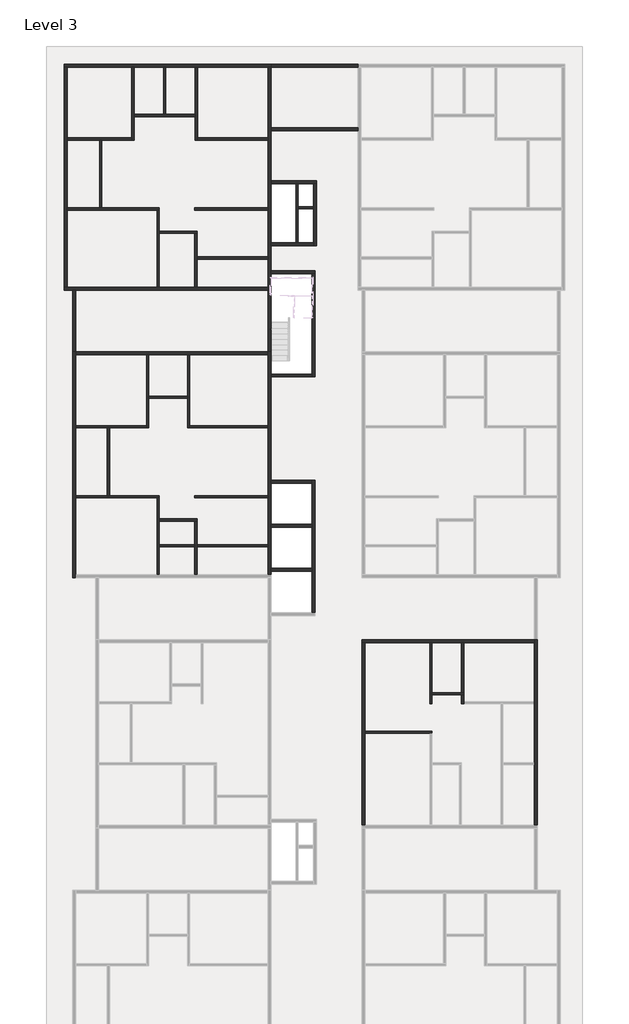
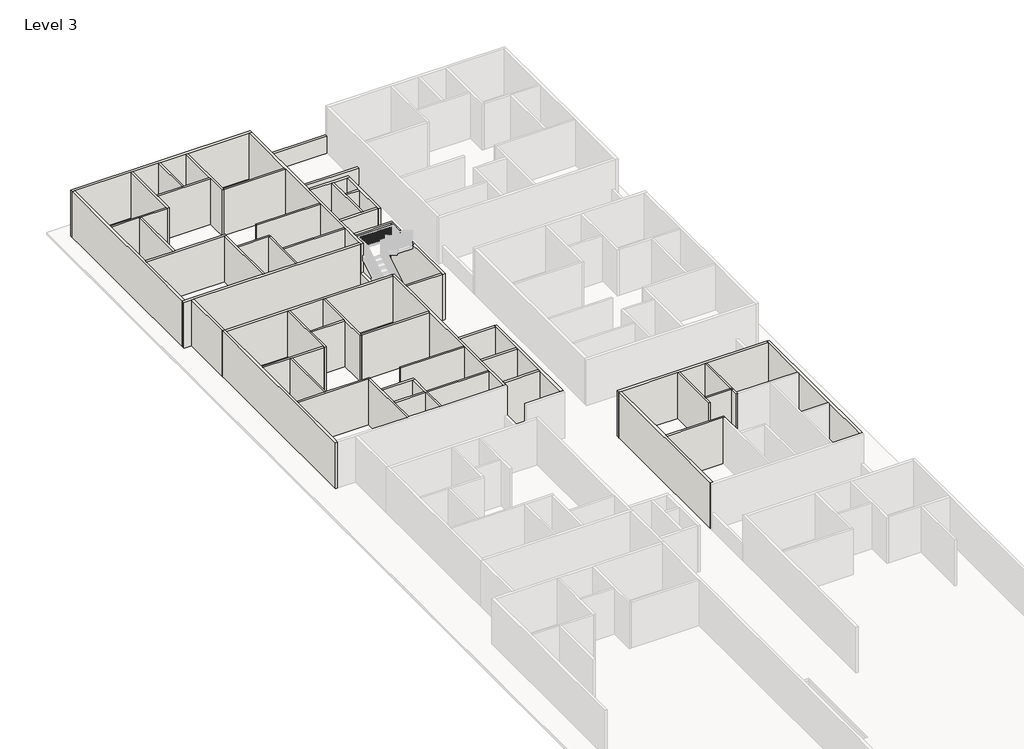
# One storey, part 3 of 8: 57 walls.
"""IFC4 building model written with IfcOpenShell, lengths in millimetres."""

from ifc_helpers import new_model, si_unit, frame, origin, place, context, project, spatial, polyline, outline, extrude, faceted_brep, element, save

model = new_model("IFC4")

# Units and contexts
model_context = context("Model", 3, world=origin())
ifc_project = project(units=[si_unit("LENGTHUNIT", "METRE", prefix="MILLI")], contexts=[model_context])

# Site, building, storey
site = spatial("IfcSite", under=ifc_project)
building = spatial("IfcBuilding", under=site)
storey = spatial("IfcBuildingStorey", under=building, Name="Level 3", Elevation=31330.6172466)

# Walls
placement = place(None, origin())
element("IfcWall", 1, ObjectType="4.5\"", at=placement, inside=storey, context=model_context, shape_type="Brep", body=[
    faceted_brep([(-10818.3415084, 35031.1216096, 31330.6172466), (-10818.3415084, 31373.5216096, 31330.6172466), (-10818.3415084, 31259.2216096, 31330.6172466), (-10818.3415084, 31259.2216096, 34378.6172466), (-10818.3415084, 31373.5216096, 34378.6172466), (-10818.3415084, 35031.1216096, 34378.6172466), (-10704.0415084, 35031.1216096, 31330.6172466), (-10704.0415084, 35031.1216096, 34378.6172466), (-10704.0415084, 32592.7216096, 34378.6172466), (-10704.0415084, 32478.4216096, 34378.6172466), (-10704.0415084, 31259.2216096, 34378.6172466), (-10704.0415084, 31259.2216096, 31330.6172466), (-10704.0415084, 32478.4216096, 31330.6172466), (-10704.0415084, 32592.7216096, 31330.6172466)], [[[0, 1, 2, 3, 4, 5]], [[6, 7, 8, 9, 10, 11, 12, 13]], [[2, 1, 0, 6, 13, 12, 11]], [[0, 5, 7, 6]], [[3, 2, 11, 10]], [[5, 4, 3, 10, 9, 8, 7]]]),
])
element("IfcWall", 2, ObjectType="4.5\"", at=placement, inside=storey, context=model_context, shape_type="Brep", body=[
    faceted_brep([(-10818.3415084, 31373.5216096, 31330.6172466), (-14171.1415084, 31373.5216096, 31330.6172466), (-14171.1415084, 31373.5216096, 34378.6172466), (-10818.3415084, 31373.5216096, 34378.6172466), (-10818.3415084, 31259.2216096, 31330.6172466), (-10818.3415084, 31259.2216096, 34378.6172466), (-12380.4415084, 31259.2216096, 34378.6172466), (-12494.7415084, 31259.2216096, 34378.6172466), (-14171.1415084, 31259.2216096, 34378.6172466), (-14171.1415084, 31259.2216096, 31330.6172466), (-12494.7415084, 31259.2216096, 31330.6172466), (-12380.4415084, 31259.2216096, 31330.6172466)], [[[0, 1, 2, 3]], [[4, 5, 6, 7, 8, 9, 10, 11]], [[1, 0, 4, 11, 10, 9]], [[0, 3, 5, 4]], [[2, 1, 9, 8]], [[3, 2, 8, 7, 6, 5]]]),
])
element("IfcWall", 3, ObjectType="4.5\"", at=placement, inside=storey, context=model_context, shape_type="SweptSolid", body=[
    extrude(outline(polyline([(-12494.7415084, 27754.0216096), (-12494.7415084, 31259.2216096), (-12380.4415084, 31259.2216096), (-12380.4415084, 27754.0216096), (-12494.7415084, 27754.0216096)])), frame((0.0, 0.0, 31330.6172466), z_axis=(0.0, 0.0, 1.0), x_axis=(1.0, 0.0, 0.0)), (0.0, 0.0, 1.0), 3048.0),
])
element("IfcWall", 4, ObjectType="4.5\"", at=placement, inside=storey, context=model_context, shape_type="Brep", body=[
    faceted_brep([(-14171.1415084, 27639.7216096, 31330.6172466), (-9510.2415084, 27639.7216096, 31330.6172466), (-9395.9415084, 27639.7216096, 31330.6172466), (-9395.9415084, 27639.7216096, 34378.6172466), (-9510.2415084, 27639.7216096, 34378.6172466), (-14171.1415084, 27639.7216096, 34378.6172466), (-14171.1415084, 27754.0216096, 31330.6172466), (-14171.1415084, 27754.0216096, 34378.6172466), (-12494.7415084, 27754.0216096, 34378.6172466), (-12380.4415084, 27754.0216096, 34378.6172466), (-9395.9415084, 27754.0216096, 34378.6172466), (-9395.9415084, 27754.0216096, 31330.6172466), (-12380.4415084, 27754.0216096, 31330.6172466), (-12494.7415084, 27754.0216096, 31330.6172466)], [[[0, 1, 2, 3, 4, 5]], [[6, 7, 8, 9, 10, 11, 12, 13]], [[2, 1, 0, 6, 13, 12, 11]], [[0, 5, 7, 6]], [[3, 2, 11, 10]], [[5, 4, 3, 10, 9, 8, 7]]]),
])
element("IfcWall", 5, ObjectType="4.5\"", at=placement, inside=storey, context=model_context, shape_type="Brep", body=[
    faceted_brep([(-9510.2415084, 27639.7216096, 31330.6172466), (-9510.2415084, 23651.9216096, 31330.6172466), (-9510.2415084, 23651.9216096, 34378.6172466), (-9510.2415084, 27639.7216096, 34378.6172466), (-9395.9415084, 27639.7216096, 31330.6172466), (-9395.9415084, 27639.7216096, 34378.6172466), (-9395.9415084, 26547.5216096, 34378.6172466), (-9395.9415084, 26433.2216096, 34378.6172466), (-9395.9415084, 23651.9216096, 34378.6172466), (-9395.9415084, 23651.9216096, 31330.6172466), (-9395.9415084, 26433.2216096, 31330.6172466), (-9395.9415084, 26547.5216096, 31330.6172466)], [[[0, 1, 2, 3]], [[4, 5, 6, 7, 8, 9, 10, 11]], [[1, 0, 4, 11, 10, 9]], [[0, 3, 5, 4]], [[2, 1, 9, 8]], [[3, 2, 8, 7, 6, 5]]]),
])
element("IfcWall", 6, ObjectType="4.5\"", at=placement, inside=storey, context=model_context, shape_type="Brep", body=[
    faceted_brep([(-9395.9415084, 26433.2216096, 31330.6172466), (-7567.1415084, 26433.2216096, 31330.6172466), (-7452.8415084, 26433.2216096, 31330.6172466), (-7452.8415084, 26433.2216096, 34378.6172466), (-7567.1415084, 26433.2216096, 34378.6172466), (-9395.9415084, 26433.2216096, 34378.6172466), (-9395.9415084, 26547.5216096, 31330.6172466), (-9395.9415084, 26547.5216096, 34378.6172466), (-7452.8415084, 26547.5216096, 34378.6172466), (-7452.8415084, 26547.5216096, 31330.6172466)], [[[0, 1, 2, 3, 4, 5]], [[6, 7, 8, 9]], [[2, 1, 0, 6, 9]], [[0, 5, 7, 6]], [[3, 2, 9, 8]], [[5, 4, 3, 8, 7]]]),
])
element("IfcWall", 7, ObjectType="4.5\"", at=placement, inside=storey, context=model_context, shape_type="Brep", body=[
    faceted_brep([(-7567.1415084, 26433.2216096, 31330.6172466), (-7567.1415084, 23651.9216096, 31330.6172466), (-7567.1415084, 23651.9216096, 34378.6172466), (-7567.1415084, 26433.2216096, 34378.6172466), (-7452.8415084, 26433.2216096, 31330.6172466), (-7452.8415084, 26433.2216096, 34378.6172466), (-7452.8415084, 25214.0216096, 34378.6172466), (-7452.8415084, 25099.7216096, 34378.6172466), (-7452.8415084, 23651.9216096, 34378.6172466), (-7452.8415084, 23651.9216096, 31330.6172466), (-7452.8415084, 25099.7216096, 31330.6172466), (-7452.8415084, 25214.0216096, 31330.6172466)], [[[0, 1, 2, 3]], [[4, 5, 6, 7, 8, 9, 10, 11]], [[1, 0, 4, 11, 10, 9]], [[0, 3, 5, 4]], [[2, 1, 9, 8]], [[3, 2, 8, 7, 6, 5]]]),
])
element("IfcWall", 8, ObjectType="4.5\"", at=placement, inside=storey, context=model_context, shape_type="SweptSolid", body=[
    extrude(outline(polyline([(-7452.8415084, 25214.0216096), (-3769.8415084, 25214.0216096), (-3769.8415084, 25099.7216096), (-7452.8415084, 25099.7216096), (-7452.8415084, 25214.0216096)])), frame((0.0, 0.0, 31330.6172466), z_axis=(0.0, 0.0, 1.0), x_axis=(1.0, 0.0, 0.0)), (0.0, 0.0, 1.0), 3048.0),
])
element("IfcWall", 9, ObjectType="4.5\"", at=placement, inside=storey, context=model_context, shape_type="SweptSolid", body=[
    extrude(outline(polyline([(-3769.8415084, 27639.7216096), (-7567.1415084, 27639.7216096), (-7567.1415084, 27754.0216096), (-3769.8415084, 27754.0216096), (-3769.8415084, 27639.7216096)])), frame((0.0, 0.0, 31330.6172466), z_axis=(0.0, 0.0, 1.0), x_axis=(1.0, 0.0, 0.0)), (0.0, 0.0, 1.0), 3048.0),
])
element("IfcWall", 10, ObjectType="4.5\"", at=placement, inside=storey, context=model_context, shape_type="Brep", body=[
    faceted_brep([(-10704.0415084, 32478.4216096, 31330.6172466), (-7541.7415084, 32478.4216096, 31330.6172466), (-7541.7415084, 32478.4216096, 34378.6172466), (-10704.0415084, 32478.4216096, 34378.6172466), (-10704.0415084, 32592.7216096, 31330.6172466), (-10704.0415084, 32592.7216096, 34378.6172466), (-9180.0415084, 32592.7216096, 34378.6172466), (-9065.7415084, 32592.7216096, 34378.6172466), (-7541.7415084, 32592.7216096, 34378.6172466), (-7541.7415084, 32592.7216096, 31330.6172466), (-9065.7415084, 32592.7216096, 31330.6172466), (-9180.0415084, 32592.7216096, 31330.6172466)], [[[0, 1, 2, 3]], [[4, 5, 6, 7, 8, 9, 10, 11]], [[1, 0, 4, 11, 10, 9]], [[0, 3, 5, 4]], [[2, 1, 9, 8]], [[3, 2, 8, 7, 6, 5]]]),
])
element("IfcWall", 11, ObjectType="4.5\"", at=placement, inside=storey, context=model_context, shape_type="SweptSolid", body=[
    extrude(outline(polyline([(-9180.0415084, 32592.7216096), (-9180.0415084, 35031.1216096), (-9065.7415084, 35031.1216096), (-9065.7415084, 32592.7216096), (-9180.0415084, 32592.7216096)])), frame((0.0, 0.0, 31330.6172466), z_axis=(0.0, 0.0, 1.0), x_axis=(1.0, 0.0, 0.0)), (0.0, 0.0, 1.0), 3048.0),
])
element("IfcWall", 12, ObjectType="4.5\"", at=placement, inside=storey, context=model_context, shape_type="Brep", body=[
    faceted_brep([(-7541.7415084, 35031.1216096, 31330.6172466), (-7541.7415084, 32592.7216096, 31330.6172466), (-7541.7415084, 32478.4216096, 31330.6172466), (-7541.7415084, 31259.2216096, 31330.6172466), (-7541.7415084, 31259.2216096, 34378.6172466), (-7541.7415084, 32478.4216096, 34378.6172466), (-7541.7415084, 32592.7216096, 34378.6172466), (-7541.7415084, 35031.1216096, 34378.6172466), (-7427.4415084, 35031.1216096, 31330.6172466), (-7427.4415084, 35031.1216096, 34378.6172466), (-7427.4415084, 31373.5216096, 34378.6172466), (-7427.4415084, 31259.2216096, 34378.6172466), (-7427.4415084, 31259.2216096, 31330.6172466), (-7427.4415084, 31373.5216096, 31330.6172466)], [[[0, 1, 2, 3, 4, 5, 6, 7]], [[8, 9, 10, 11, 12, 13]], [[3, 2, 1, 0, 8, 13, 12]], [[0, 7, 9, 8]], [[4, 3, 12, 11]], [[7, 6, 5, 4, 11, 10, 9]]]),
])
element("IfcWall", 13, ObjectType="4.5\"", at=placement, inside=storey, context=model_context, shape_type="SweptSolid", body=[
    extrude(outline(polyline([(-3769.8415084, 31259.2216096), (-7427.4415084, 31259.2216096), (-7427.4415084, 31373.5216096), (-3769.8415084, 31373.5216096), (-3769.8415084, 31259.2216096)])), frame((0.0, 0.0, 31330.6172466), z_axis=(0.0, 0.0, 1.0), x_axis=(1.0, 0.0, 0.0)), (0.0, 0.0, 1.0), 3048.0),
])
element("IfcWall", 14, ObjectType="4.5\"", at=placement, inside=storey, context=model_context, shape_type="Brep", body=[
    faceted_brep([(-10061.4044854, 20146.7216096, 31330.6172466), (-10061.4044854, 16489.1216096, 31330.6172466), (-10061.4044854, 16374.8216096, 31330.6172466), (-10061.4044854, 16374.8216096, 34378.6172466), (-10061.4044854, 16489.1216096, 34378.6172466), (-10061.4044854, 20146.7216096, 34378.6172466), (-9947.1044854, 20146.7216096, 31330.6172466), (-9947.1044854, 20146.7216096, 34378.6172466), (-9947.1044854, 18013.1216096, 34378.6172466), (-9947.1044854, 17898.8216096, 34378.6172466), (-9947.1044854, 16374.8216096, 34378.6172466), (-9947.1044854, 16374.8216096, 31330.6172466), (-9947.1044854, 17898.8216096, 31330.6172466), (-9947.1044854, 18013.1216096, 31330.6172466)], [[[0, 1, 2, 3, 4, 5]], [[6, 7, 8, 9, 10, 11, 12, 13]], [[2, 1, 0, 6, 13, 12, 11]], [[0, 5, 7, 6]], [[3, 2, 11, 10]], [[5, 4, 3, 10, 9, 8, 7]]]),
])
element("IfcWall", 15, ObjectType="4.5\"", at=placement, inside=storey, context=model_context, shape_type="Brep", body=[
    faceted_brep([(-10061.4044854, 16489.1216096, 31330.6172466), (-13719.0044854, 16489.1216096, 31330.6172466), (-13719.0044854, 16489.1216096, 34378.6172466), (-10061.4044854, 16489.1216096, 34378.6172466), (-10061.4044854, 16374.8216096, 31330.6172466), (-10061.4044854, 16374.8216096, 34378.6172466), (-11980.3915084, 16374.8216096, 34378.6172466), (-12094.6915084, 16374.8216096, 34378.6172466), (-13719.0044854, 16374.8216096, 34378.6172466), (-13719.0044854, 16374.8216096, 31330.6172466), (-12094.6915084, 16374.8216096, 31330.6172466), (-11980.3915084, 16374.8216096, 31330.6172466)], [[[0, 1, 2, 3]], [[4, 5, 6, 7, 8, 9, 10, 11]], [[1, 0, 4, 11, 10, 9]], [[0, 3, 5, 4]], [[2, 1, 9, 8]], [[3, 2, 8, 7, 6, 5]]]),
])
element("IfcWall", 16, ObjectType="4.5\"", at=placement, inside=storey, context=model_context, shape_type="SweptSolid", body=[
    extrude(outline(polyline([(-7940.5044854, 17898.8216096), (-9947.1044854, 17898.8216096), (-9947.1044854, 18013.1216096), (-7940.5044854, 18013.1216096), (-7940.5044854, 17898.8216096)])), frame((0.0, 0.0, 31330.6172466), z_axis=(0.0, 0.0, 1.0), x_axis=(1.0, 0.0, 0.0)), (0.0, 0.0, 1.0), 3048.0),
])
element("IfcWall", 17, ObjectType="4.5\"", at=placement, inside=storey, context=model_context, shape_type="Brep", body=[
    faceted_brep([(-7940.5044854, 20146.7216096, 31330.6172466), (-7940.5044854, 18013.1216096, 31330.6172466), (-7940.5044854, 17898.8216096, 31330.6172466), (-7940.5044854, 16374.8216096, 31330.6172466), (-7940.5044854, 16374.8216096, 34378.6172466), (-7940.5044854, 17898.8216096, 34378.6172466), (-7940.5044854, 18013.1216096, 34378.6172466), (-7940.5044854, 20146.7216096, 34378.6172466), (-7826.2044854, 20146.7216096, 31330.6172466), (-7826.2044854, 20146.7216096, 34378.6172466), (-7826.2044854, 16489.1216096, 34378.6172466), (-7826.2044854, 16374.8216096, 34378.6172466), (-7826.2044854, 16374.8216096, 31330.6172466), (-7826.2044854, 16489.1216096, 31330.6172466)], [[[0, 1, 2, 3, 4, 5, 6, 7]], [[8, 9, 10, 11, 12, 13]], [[3, 2, 1, 0, 8, 13, 12]], [[0, 7, 9, 8]], [[4, 3, 12, 11]], [[7, 6, 5, 4, 11, 10, 9]]]),
])
element("IfcWall", 18, ObjectType="4.5\"", at=placement, inside=storey, context=model_context, shape_type="SweptSolid", body=[
    extrude(outline(polyline([(-3769.8415084, 16374.8216096), (-7826.2044854, 16374.8216096), (-7826.2044854, 16489.1216096), (-3769.8415084, 16489.1216096), (-3769.8415084, 16374.8216096)])), frame((0.0, 0.0, 31330.6172466), z_axis=(0.0, 0.0, 1.0), x_axis=(1.0, 0.0, 0.0)), (0.0, 0.0, 1.0), 3048.0),
])
element("IfcWall", 19, ObjectType="4.5\"", at=placement, inside=storey, context=model_context, shape_type="SweptSolid", body=[
    extrude(outline(polyline([(-12094.6915084, 12869.6216096), (-12094.6915084, 16374.8216096), (-11980.3915084, 16374.8216096), (-11980.3915084, 12869.6216096), (-12094.6915084, 12869.6216096)])), frame((0.0, 0.0, 31330.6172466), z_axis=(0.0, 0.0, 1.0), x_axis=(1.0, 0.0, 0.0)), (0.0, 0.0, 1.0), 3048.0),
])
element("IfcWall", 20, ObjectType="4.5\"", at=placement, inside=storey, context=model_context, shape_type="Brep", body=[
    faceted_brep([(-13719.0044854, 12755.3216096, 31330.6172466), (-9510.2415084, 12755.3216096, 31330.6172466), (-9395.9415084, 12755.3216096, 31330.6172466), (-9395.9415084, 12755.3216096, 34378.6172466), (-9510.2415084, 12755.3216096, 34378.6172466), (-13719.0044854, 12755.3216096, 34378.6172466), (-13719.0044854, 12869.6216096, 31330.6172466), (-13719.0044854, 12869.6216096, 34378.6172466), (-12094.6915084, 12869.6216096, 34378.6172466), (-11980.3915084, 12869.6216096, 34378.6172466), (-9395.9415084, 12869.6216096, 34378.6172466), (-9395.9415084, 12869.6216096, 31330.6172466), (-11980.3915084, 12869.6216096, 31330.6172466), (-12094.6915084, 12869.6216096, 31330.6172466)], [[[0, 1, 2, 3, 4, 5]], [[6, 7, 8, 9, 10, 11, 12, 13]], [[2, 1, 0, 6, 13, 12, 11]], [[0, 5, 7, 6]], [[3, 2, 11, 10]], [[5, 4, 3, 10, 9, 8, 7]]]),
])
element("IfcWall", 21, ObjectType="4.5\"", at=placement, inside=storey, context=model_context, shape_type="Brep", body=[
    faceted_brep([(-9510.2415084, 12755.3216096, 31330.6172466), (-9510.2415084, 8767.5216096, 31330.6172466), (-9510.2415084, 8767.5216096, 34378.6172466), (-9510.2415084, 12755.3216096, 34378.6172466), (-9395.9415084, 12755.3216096, 31330.6172466), (-9395.9415084, 12755.3216096, 34378.6172466), (-9395.9415084, 11663.1216096, 34378.6172466), (-9395.9415084, 11548.8216096, 34378.6172466), (-9395.9415084, 10329.6216096, 34378.6172466), (-9395.9415084, 10215.3216096, 34378.6172466), (-9395.9415084, 8767.5216096, 34378.6172466), (-9395.9415084, 8767.5216096, 31330.6172466), (-9395.9415084, 10215.3216096, 31330.6172466), (-9395.9415084, 10329.6216096, 31330.6172466), (-9395.9415084, 11548.8216096, 31330.6172466), (-9395.9415084, 11663.1216096, 31330.6172466)], [[[0, 1, 2, 3]], [[4, 5, 6, 7, 8, 9, 10, 11, 12, 13, 14, 15]], [[1, 0, 4, 15, 14, 13, 12, 11]], [[0, 3, 5, 4]], [[2, 1, 11, 10]], [[3, 2, 10, 9, 8, 7, 6, 5]]]),
])
element("IfcWall", 22, ObjectType="4.5\"", at=placement, inside=storey, context=model_context, shape_type="SweptSolid", body=[
    extrude(outline(polyline([(-7567.1415084, 10215.3216096), (-9395.9415084, 10215.3216096), (-9395.9415084, 10329.6216096), (-7567.1415084, 10329.6216096), (-7567.1415084, 10215.3216096)])), frame((0.0, 0.0, 31330.6172466), z_axis=(0.0, 0.0, 1.0), x_axis=(1.0, 0.0, 0.0)), (0.0, 0.0, 1.0), 3048.0),
])
element("IfcWall", 23, ObjectType="4.5\"", at=placement, inside=storey, context=model_context, shape_type="Brep", body=[
    faceted_brep([(-9395.9415084, 11548.8216096, 31330.6172466), (-7567.1415084, 11548.8216096, 31330.6172466), (-7452.8415084, 11548.8216096, 31330.6172466), (-7452.8415084, 11548.8216096, 34378.6172466), (-7567.1415084, 11548.8216096, 34378.6172466), (-9395.9415084, 11548.8216096, 34378.6172466), (-9395.9415084, 11663.1216096, 31330.6172466), (-9395.9415084, 11663.1216096, 34378.6172466), (-7452.8415084, 11663.1216096, 34378.6172466), (-7452.8415084, 11663.1216096, 31330.6172466)], [[[0, 1, 2, 3, 4, 5]], [[6, 7, 8, 9]], [[2, 1, 0, 6, 9]], [[0, 5, 7, 6]], [[3, 2, 9, 8]], [[5, 4, 3, 8, 7]]]),
])
element("IfcWall", 24, ObjectType="4.5\"", at=placement, inside=storey, context=model_context, shape_type="Brep", body=[
    faceted_brep([(-7567.1415084, 11548.8216096, 31330.6172466), (-7567.1415084, 10329.6216096, 31330.6172466), (-7567.1415084, 10215.3216096, 31330.6172466), (-7567.1415084, 8767.5216096, 31330.6172466), (-7567.1415084, 8767.5216096, 34378.6172466), (-7567.1415084, 10215.3216096, 34378.6172466), (-7567.1415084, 10329.6216096, 34378.6172466), (-7567.1415084, 11548.8216096, 34378.6172466), (-7452.8415084, 11548.8216096, 31330.6172466), (-7452.8415084, 11548.8216096, 34378.6172466), (-7452.8415084, 10329.6216096, 34378.6172466), (-7452.8415084, 10215.3216096, 34378.6172466), (-7452.8415084, 8767.5216096, 34378.6172466), (-7452.8415084, 8767.5216096, 31330.6172466), (-7452.8415084, 10215.3216096, 31330.6172466), (-7452.8415084, 10329.6216096, 31330.6172466)], [[[0, 1, 2, 3, 4, 5, 6, 7]], [[8, 9, 10, 11, 12, 13, 14, 15]], [[3, 2, 1, 0, 8, 15, 14, 13]], [[0, 7, 9, 8]], [[4, 3, 13, 12]], [[7, 6, 5, 4, 12, 11, 10, 9]]]),
])
element("IfcWall", 25, ObjectType="4.5\"", at=placement, inside=storey, context=model_context, shape_type="SweptSolid", body=[
    extrude(outline(polyline([(-3769.8415084, 10215.3216096), (-7452.8415084, 10215.3216096), (-7452.8415084, 10329.6216096), (-3769.8415084, 10329.6216096), (-3769.8415084, 10215.3216096)])), frame((0.0, 0.0, 31330.6172466), z_axis=(0.0, 0.0, 1.0), x_axis=(1.0, 0.0, 0.0)), (0.0, 0.0, 1.0), 3048.0),
])
element("IfcWall", 26, ObjectType="4.5\"", at=placement, inside=storey, context=model_context, shape_type="SweptSolid", body=[
    extrude(outline(polyline([(-3769.8415084, 12755.3216096), (-7567.1415084, 12755.3216096), (-7567.1415084, 12869.6216096), (-3769.8415084, 12869.6216096), (-3769.8415084, 12755.3216096)])), frame((0.0, 0.0, 31330.6172466), z_axis=(0.0, 0.0, 1.0), x_axis=(1.0, 0.0, 0.0)), (0.0, 0.0, 1.0), 3048.0),
])
element("IfcWall", 27, ObjectType="4.5\"", at=placement, inside=storey, context=model_context, shape_type="Brep", body=[
    faceted_brep([(1259.3584916, 572.7745083, 31330.6172466), (4610.8714687, 572.7745083, 31330.6172466), (4725.1714687, 572.7745083, 31330.6172466), (4725.1714687, 572.7745083, 34378.6172466), (4610.8714687, 572.7745083, 34378.6172466), (1259.3584916, 572.7745083, 34378.6172466), (1259.3584916, 687.0745083, 31330.6172466), (1259.3584916, 687.0745083, 34378.6172466), (4725.1714687, 687.0745083, 34378.6172466), (4725.1714687, 687.0745083, 31330.6172466)], [[[0, 1, 2, 3, 4, 5]], [[6, 7, 8, 9]], [[2, 1, 0, 6, 9]], [[0, 5, 7, 6]], [[3, 2, 9, 8]], [[5, 4, 3, 8, 7]]]),
])
element("IfcWall", 28, ObjectType="4.5\"", at=placement, inside=storey, context=model_context, shape_type="Brep", body=[
    faceted_brep([(4610.8714687, 5262.3216096, 31330.6172466), (4610.8714687, 2100.0216096, 31330.6172466), (4610.8714687, 2100.0216096, 34378.6172466), (4610.8714687, 5262.3216096, 34378.6172466), (4725.1714687, 5262.3216096, 31330.6172466), (4725.1714687, 5262.3216096, 34378.6172466), (4725.1714687, 2671.5216096, 34378.6172466), (4725.1714687, 2557.2216096, 34378.6172466), (4725.1714687, 2100.0216096, 34378.6172466), (4725.1714687, 2100.0216096, 31330.6172466), (4725.1714687, 2557.2216096, 31330.6172466), (4725.1714687, 2671.5216096, 31330.6172466)], [[[0, 1, 2, 3]], [[4, 5, 6, 7, 8, 9, 10, 11]], [[1, 0, 4, 11, 10, 9]], [[2, 1, 9, 8]], [[0, 3, 5, 4]], [[3, 2, 8, 7, 6, 5]]]),
])
element("IfcWall", 29, ObjectType="4.5\"", at=placement, inside=storey, context=model_context, shape_type="Brep", body=[
    faceted_brep([(4725.1714687, 2557.2216096, 31330.6172466), (6249.1714687, 2557.2216096, 31330.6172466), (6363.4714687, 2557.2216096, 31330.6172466), (6363.4714687, 2557.2216096, 34378.6172466), (6249.1714687, 2557.2216096, 34378.6172466), (4725.1714687, 2557.2216096, 34378.6172466), (4725.1714687, 2671.5216096, 31330.6172466), (4725.1714687, 2671.5216096, 34378.6172466), (6249.1714687, 2671.5216096, 34378.6172466), (6363.4714687, 2671.5216096, 34378.6172466), (6363.4714687, 2671.5216096, 31330.6172466), (6249.1714687, 2671.5216096, 31330.6172466)], [[[0, 1, 2, 3, 4, 5]], [[6, 7, 8, 9, 10, 11]], [[2, 1, 0, 6, 11, 10]], [[0, 5, 7, 6]], [[3, 2, 10, 9]], [[5, 4, 3, 9, 8, 7]]]),
])
element("IfcWall", 30, ObjectType="4.5\"", at=placement, inside=storey, context=model_context, shape_type="SweptSolid", body=[
    extrude(outline(polyline([(6363.4714687, 5262.3216096), (6363.4714687, 2671.5216096), (6249.1714687, 2671.5216096), (6249.1714687, 5262.3216096), (6363.4714687, 5262.3216096)])), frame((0.0, 0.0, 31330.6172466), z_axis=(0.0, 0.0, 1.0), x_axis=(1.0, 0.0, 0.0)), (0.0, 0.0, 1.0), 3048.0),
])
element("IfcWall", 31, ObjectType="4.5\"", at=placement, inside=storey, context=model_context, shape_type="Brep", body=[
    faceted_brep([(6249.1714687, 2557.2216096, 31330.6172466), (6249.1714687, 2100.0216096, 31330.6172466), (6249.1714687, 2100.0216096, 34378.6172466), (6249.1714687, 2557.2216096, 34378.6172466), (6363.4714687, 2557.2216096, 31330.6172466), (6363.4714687, 2557.2216096, 34378.6172466), (6363.4714687, 2214.3216096, 34378.6172466), (6363.4714687, 2100.0216096, 34378.6172466), (6363.4714687, 2100.0216096, 31330.6172466), (6363.4714687, 2214.3216096, 31330.6172466)], [[[0, 1, 2, 3]], [[4, 5, 6, 7, 8, 9]], [[1, 0, 4, 9, 8]], [[0, 3, 5, 4]], [[2, 1, 8, 7]], [[3, 2, 7, 6, 5]]]),
])
element("IfcWall", 32, ObjectType="4.5\"", at=placement, inside=storey, context=model_context, shape_type="Brep", body=[
    faceted_brep([(-2321.9738684, 29000.0900967, 31330.6172466), (-2321.9738684, 25952.0900967, 31330.6172466), (-2321.9738684, 25952.0900967, 34378.6172466), (-2321.9738684, 29000.0900967, 34378.6172466), (-2207.6738684, 29000.0900967, 31330.6172466), (-2207.6738684, 29000.0900967, 34378.6172466), (-2207.6738684, 27820.8172885, 34378.6172466), (-2207.6738684, 27706.5172885, 34378.6172466), (-2207.6738684, 25952.0900967, 34378.6172466), (-2207.6738684, 25952.0900967, 31330.6172466), (-2207.6738684, 27706.5172885, 31330.6172466), (-2207.6738684, 27820.8172885, 31330.6172466)], [[[0, 1, 2, 3]], [[4, 5, 6, 7, 8, 9, 10, 11]], [[1, 0, 4, 11, 10, 9]], [[3, 2, 8, 7, 6, 5]], [[0, 3, 5, 4]], [[2, 1, 9, 8]]]),
])
element("IfcWall", 33, ObjectType="4.5\"", at=placement, inside=storey, context=model_context, shape_type="SweptSolid", body=[
    extrude(outline(polyline([(-2207.6738684, 27820.8172885), (-1407.6415084, 27820.8172885), (-1407.6415084, 27706.5172885), (-2207.6738684, 27706.5172885), (-2207.6738684, 27820.8172885)])), frame((0.0, 0.0, 31330.6172466), z_axis=(0.0, 0.0, 1.0), x_axis=(1.0, 0.0, 0.0)), (0.0, 0.0, 1.0), 3048.0),
])
element("IfcWall", 34, ObjectType="6\"", at=placement, inside=storey, context=model_context, shape_type="Brep", body=[
    faceted_brep([(-14323.5415084, 35031.1216096, 31330.6172466), (-14171.1415084, 35031.1216096, 31330.6172466), (-10818.3415084, 35031.1216096, 31330.6172466), (-10704.0415084, 35031.1216096, 31330.6172466), (-9180.0415084, 35031.1216096, 31330.6172466), (-9065.7415084, 35031.1216096, 31330.6172466), (-7541.7415084, 35031.1216096, 31330.6172466), (-7427.4415084, 35031.1216096, 31330.6172466), (-3769.8415084, 35031.1216096, 31330.6172466), (-3617.4415084, 35031.1216096, 31330.6172466), (-3617.4415084, 35031.1216096, 34378.6172466), (-3769.8415084, 35031.1216096, 34378.6172466), (-7427.4415084, 35031.1216096, 34378.6172466), (-7541.7415084, 35031.1216096, 34378.6172466), (-9065.7415084, 35031.1216096, 34378.6172466), (-9180.0415084, 35031.1216096, 34378.6172466), (-10704.0415084, 35031.1216096, 34378.6172466), (-10818.3415084, 35031.1216096, 34378.6172466), (-14171.1415084, 35031.1216096, 34378.6172466), (-14323.5415084, 35031.1216096, 34378.6172466), (-14323.5415084, 35183.5216096, 31330.6172466), (-14323.5415084, 35183.5216096, 34378.6172466), (-3617.4415084, 35183.5216096, 34378.6172466), (-3617.4415084, 35183.5216096, 31330.6172466)], [[[0, 1, 2, 3, 4, 5, 6, 7, 8, 9, 10, 11, 12, 13, 14, 15, 16, 17, 18, 19]], [[20, 21, 22, 23]], [[9, 8, 7, 6, 5, 4, 3, 2, 1, 0, 20, 23]], [[0, 19, 21, 20]], [[9, 23, 22, 10]], [[19, 18, 17, 16, 15, 14, 13, 12, 11, 10, 22, 21]]]),
])
element("IfcWall", 35, ObjectType="6\"", at=placement, inside=storey, context=model_context, shape_type="Brep", body=[
    faceted_brep([(-3769.8415084, 35031.1216096, 34378.6172466), (-3769.8415084, 35031.1216096, 31330.6172466), (-3769.8415084, 31373.5216096, 31330.6172466), (-3769.8415084, 31259.2216096, 31330.6172466), (-3769.8415084, 27754.0216096, 31330.6172466), (-3769.8415084, 27639.7216096, 31330.6172466), (-3769.8415084, 25214.0216096, 31330.6172466), (-3769.8415084, 25099.7216096, 31330.6172466), (-3769.8415084, 23651.9216096, 31330.6172466), (-3769.8415084, 23499.5216096, 31330.6172466), (-3769.8415084, 23499.5216096, 34378.6172466), (-3769.8415084, 23651.9216096, 34378.6172466), (-3769.8415084, 25099.7216096, 34378.6172466), (-3769.8415084, 25214.0216096, 34378.6172466), (-3769.8415084, 27639.7216096, 34378.6172466), (-3769.8415084, 27754.0216096, 34378.6172466), (-3769.8415084, 31259.2216096, 34378.6172466), (-3769.8415084, 31373.5216096, 34378.6172466), (-3617.4415084, 35031.1216096, 31330.6172466), (-3617.4415084, 35031.1216096, 34378.6172466), (-3617.4415084, 29152.4900967, 34378.6172466), (-3617.4415084, 29000.0900967, 34378.6172466), (-3617.4415084, 25952.0900967, 34378.6172466), (-3617.4415084, 25799.6900967, 34378.6172466), (-3617.4415084, 24490.1216096, 34378.6172466), (-3617.4415084, 24337.7216096, 34378.6172466), (-3617.4415084, 23499.5216096, 34378.6172466), (-3617.4415084, 23499.5216096, 31330.6172466), (-3617.4415084, 24337.7216096, 31330.6172466), (-3617.4415084, 24490.1216096, 31330.6172466), (-3617.4415084, 25799.6900967, 31330.6172466), (-3617.4415084, 25952.0900967, 31330.6172466), (-3617.4415084, 29000.0900967, 31330.6172466), (-3617.4415084, 29152.4900967, 31330.6172466), (-3617.4415084, 31744.9197155, 31330.6172466), (-3617.4415084, 31897.3197155, 31330.6172466)], [[[0, 1, 2, 3, 4, 5, 6, 7, 8, 9, 10, 11, 12, 13, 14, 15, 16, 17]], [[18, 19, 20, 21, 22, 23, 24, 25, 26, 27, 28, 29, 30, 31, 32, 33, 34, 35]], [[9, 8, 7, 6, 5, 4, 3, 2, 1, 18, 35, 34, 33, 32, 31, 30, 29, 28, 27]], [[0, 19, 18, 1]], [[9, 27, 26, 10]], [[0, 17, 16, 15, 14, 13, 12, 11, 10, 26, 25, 24, 23, 22, 21, 20, 19]]]),
])
element("IfcWall", 36, ObjectType="6\"", at=placement, inside=storey, context=model_context, shape_type="Brep", body=[
    faceted_brep([(-3769.8415084, 23651.9216096, 34378.6172466), (-3769.8415084, 23651.9216096, 31330.6172466), (-7452.8415084, 23651.9216096, 31330.6172466), (-7567.1415084, 23651.9216096, 31330.6172466), (-9395.9415084, 23651.9216096, 31330.6172466), (-9510.2415084, 23651.9216096, 31330.6172466), (-14171.1415084, 23651.9216096, 31330.6172466), (-14323.5415084, 23651.9216096, 31330.6172466), (-14323.5415084, 23651.9216096, 34378.6172466), (-14171.1415084, 23651.9216096, 34378.6172466), (-9510.2415084, 23651.9216096, 34378.6172466), (-9395.9415084, 23651.9216096, 34378.6172466), (-7567.1415084, 23651.9216096, 34378.6172466), (-7452.8415084, 23651.9216096, 34378.6172466), (-3769.8415084, 23499.5216096, 31330.6172466), (-3769.8415084, 23499.5216096, 34378.6172466), (-13719.0044854, 23499.5216096, 34378.6172466), (-13871.4044854, 23499.5216096, 34378.6172466), (-14323.5415084, 23499.5216096, 34378.6172466), (-14323.5415084, 23499.5216096, 31330.6172466), (-13871.4044854, 23499.5216096, 31330.6172466), (-13719.0044854, 23499.5216096, 31330.6172466)], [[[0, 1, 2, 3, 4, 5, 6, 7, 8, 9, 10, 11, 12, 13]], [[14, 15, 16, 17, 18, 19, 20, 21]], [[7, 6, 5, 4, 3, 2, 1, 14, 21, 20, 19]], [[8, 7, 19, 18]], [[0, 15, 14, 1]], [[0, 13, 12, 11, 10, 9, 8, 18, 17, 16, 15]]]),
])
element("IfcWall", 37, ObjectType="6\"", at=placement, inside=storey, context=model_context, shape_type="Brep", body=[
    faceted_brep([(-14171.1415084, 23651.9216096, 31330.6172466), (-14171.1415084, 27639.7216096, 31330.6172466), (-14171.1415084, 27754.0216096, 31330.6172466), (-14171.1415084, 31259.2216096, 31330.6172466), (-14171.1415084, 31373.5216096, 31330.6172466), (-14171.1415084, 35031.1216096, 31330.6172466), (-14171.1415084, 35031.1216096, 34378.6172466), (-14171.1415084, 31373.5216096, 34378.6172466), (-14171.1415084, 31259.2216096, 34378.6172466), (-14171.1415084, 27754.0216096, 34378.6172466), (-14171.1415084, 27639.7216096, 34378.6172466), (-14171.1415084, 23651.9216096, 34378.6172466), (-14323.5415084, 23651.9216096, 31330.6172466), (-14323.5415084, 23651.9216096, 34378.6172466), (-14323.5415084, 35031.1216096, 34378.6172466), (-14323.5415084, 35031.1216096, 31330.6172466)], [[[0, 1, 2, 3, 4, 5, 6, 7, 8, 9, 10, 11]], [[12, 13, 14, 15]], [[5, 4, 3, 2, 1, 0, 12, 15]], [[6, 5, 15, 14]], [[0, 11, 13, 12]], [[11, 10, 9, 8, 7, 6, 14, 13]]]),
])
element("IfcWall", 38, ObjectType="6\"", at=placement, inside=storey, context=model_context, shape_type="Brep", body=[
    faceted_brep([(-13871.4044854, 20299.1216096, 31330.6172466), (-13871.4044854, 8615.1216096, 31330.6172466), (-13871.4044854, 8615.1216096, 34378.6172466), (-13871.4044854, 20299.1216096, 34378.6172466), (-13719.0044854, 20299.1216096, 31330.6172466), (-13719.0044854, 20299.1216096, 34378.6172466), (-13719.0044854, 20146.7216096, 34378.6172466), (-13719.0044854, 16489.1216096, 34378.6172466), (-13719.0044854, 16374.8216096, 34378.6172466), (-13719.0044854, 12869.6216096, 34378.6172466), (-13719.0044854, 12755.3216096, 34378.6172466), (-13719.0044854, 8767.5216096, 34378.6172466), (-13719.0044854, 8615.1216096, 34378.6172466), (-13719.0044854, 8615.1216096, 31330.6172466), (-13719.0044854, 8767.5216096, 31330.6172466), (-13719.0044854, 12755.3216096, 31330.6172466), (-13719.0044854, 12869.6216096, 31330.6172466), (-13719.0044854, 16374.8216096, 31330.6172466), (-13719.0044854, 16489.1216096, 31330.6172466), (-13719.0044854, 20146.7216096, 31330.6172466)], [[[0, 1, 2, 3]], [[4, 5, 6, 7, 8, 9, 10, 11, 12, 13, 14, 15, 16, 17, 18, 19]], [[1, 0, 4, 19, 18, 17, 16, 15, 14, 13]], [[2, 1, 13, 12]], [[0, 3, 5, 4]], [[3, 2, 12, 11, 10, 9, 8, 7, 6, 5]]]),
])
element("IfcWall", 39, ObjectType="6\"", at=placement, inside=storey, context=model_context, shape_type="Brep", body=[
    faceted_brep([(-3617.4415084, 8767.5216096, 34378.6172466), (-3617.4415084, 8767.5216096, 31330.6172466), (-3617.4415084, 8945.2303368, 31330.6172466), (-3617.4415084, 9097.6303368, 31330.6172466), (-3617.4415084, 11231.2303368, 31330.6172466), (-3617.4415084, 11383.6303368, 31330.6172466), (-3617.4415084, 13517.2303368, 31330.6172466), (-3617.4415084, 13669.6303368, 31330.6172466), (-3617.4415084, 19003.7216096, 31330.6172466), (-3617.4415084, 19156.1216096, 31330.6172466), (-3617.4415084, 20299.1216096, 31330.6172466), (-3617.4415084, 20299.1216096, 34378.6172466), (-3617.4415084, 19156.1216096, 34378.6172466), (-3617.4415084, 19003.7216096, 34378.6172466), (-3617.4415084, 13669.6303368, 34378.6172466), (-3617.4415084, 13517.2303368, 34378.6172466), (-3617.4415084, 11383.6303368, 34378.6172466), (-3617.4415084, 11231.2303368, 34378.6172466), (-3617.4415084, 9097.6303368, 34378.6172466), (-3617.4415084, 8945.2303368, 34378.6172466), (-3769.8415084, 8767.5216096, 31330.6172466), (-3769.8415084, 8767.5216096, 34378.6172466), (-3769.8415084, 10215.3216096, 34378.6172466), (-3769.8415084, 10329.6216096, 34378.6172466), (-3769.8415084, 12755.3216096, 34378.6172466), (-3769.8415084, 12869.6216096, 34378.6172466), (-3769.8415084, 16374.8216096, 34378.6172466), (-3769.8415084, 16489.1216096, 34378.6172466), (-3769.8415084, 20146.7216096, 34378.6172466), (-3769.8415084, 20299.1216096, 34378.6172466), (-3769.8415084, 20299.1216096, 31330.6172466), (-3769.8415084, 20146.7216096, 31330.6172466), (-3769.8415084, 16489.1216096, 31330.6172466), (-3769.8415084, 16374.8216096, 31330.6172466), (-3769.8415084, 12869.6216096, 31330.6172466), (-3769.8415084, 12755.3216096, 31330.6172466), (-3769.8415084, 10329.6216096, 31330.6172466), (-3769.8415084, 10215.3216096, 31330.6172466)], [[[0, 1, 2, 3, 4, 5, 6, 7, 8, 9, 10, 11, 12, 13, 14, 15, 16, 17, 18, 19]], [[20, 21, 22, 23, 24, 25, 26, 27, 28, 29, 30, 31, 32, 33, 34, 35, 36, 37]], [[10, 9, 8, 7, 6, 5, 4, 3, 2, 1, 20, 37, 36, 35, 34, 33, 32, 31, 30]], [[10, 30, 29, 11]], [[0, 21, 20, 1]], [[0, 19, 18, 17, 16, 15, 14, 13, 12, 11, 29, 28, 27, 26, 25, 24, 23, 22, 21]]]),
])
element("IfcWall", 40, ObjectType="6\"", at=placement, inside=storey, context=model_context, shape_type="Brep", body=[
    faceted_brep([(-3769.8415084, 20299.1216096, 34378.6172466), (-3769.8415084, 20299.1216096, 31330.6172466), (-13719.0044854, 20299.1216096, 31330.6172466), (-13719.0044854, 20299.1216096, 34378.6172466), (-3769.8415084, 20146.7216096, 31330.6172466), (-3769.8415084, 20146.7216096, 34378.6172466), (-7826.2044854, 20146.7216096, 34378.6172466), (-7940.5044854, 20146.7216096, 34378.6172466), (-9947.1044854, 20146.7216096, 34378.6172466), (-10061.4044854, 20146.7216096, 34378.6172466), (-13719.0044854, 20146.7216096, 34378.6172466), (-13719.0044854, 20146.7216096, 31330.6172466), (-10061.4044854, 20146.7216096, 31330.6172466), (-9947.1044854, 20146.7216096, 31330.6172466), (-7940.5044854, 20146.7216096, 31330.6172466), (-7826.2044854, 20146.7216096, 31330.6172466)], [[[0, 1, 2, 3]], [[4, 5, 6, 7, 8, 9, 10, 11, 12, 13, 14, 15]], [[2, 1, 4, 15, 14, 13, 12, 11]], [[3, 2, 11, 10]], [[0, 5, 4, 1]], [[0, 3, 10, 9, 8, 7, 6, 5]]]),
])
element("IfcWall", 41, ObjectType="6\"", at=placement, inside=storey, context=model_context, shape_type="Brep", body=[
    faceted_brep([(10173.4714687, -4185.9344126, 34378.6172466), (10173.4714687, -4185.9344126, 31330.6172466), (10173.4714687, 5414.7216096, 31330.6172466), (10173.4714687, 5414.7216096, 34378.6172466), (10021.0714687, -4185.9344126, 31330.6172466), (10021.0714687, -4185.9344126, 34378.6172466), (10021.0714687, -1061.7344126, 34378.6172466), (10021.0714687, -947.4344126, 34378.6172466), (10021.0714687, 2100.0216096, 34378.6172466), (10021.0714687, 2214.3216096, 34378.6172466), (10021.0714687, 5262.3216096, 34378.6172466), (10021.0714687, 5414.7216096, 34378.6172466), (10021.0714687, 5414.7216096, 31330.6172466), (10021.0714687, 5262.3216096, 31330.6172466), (10021.0714687, 2214.3216096, 31330.6172466), (10021.0714687, 2100.0216096, 31330.6172466), (10021.0714687, -947.4344126, 31330.6172466), (10021.0714687, -1061.7344126, 31330.6172466)], [[[0, 1, 2, 3]], [[4, 5, 6, 7, 8, 9, 10, 11, 12, 13, 14, 15, 16, 17]], [[2, 1, 4, 17, 16, 15, 14, 13, 12]], [[2, 12, 11, 3]], [[0, 5, 4, 1]], [[0, 3, 11, 10, 9, 8, 7, 6, 5]]]),
])
element("IfcWall", 42, ObjectType="6\"", at=placement, inside=storey, context=model_context, shape_type="Brep", body=[
    faceted_brep([(10021.0714687, 5414.7216096, 34378.6172466), (10021.0714687, 5414.7216096, 31330.6172466), (1106.9584916, 5414.7216096, 31330.6172466), (1106.9584916, 5414.7216096, 34378.6172466), (10021.0714687, 5262.3216096, 31330.6172466), (10021.0714687, 5262.3216096, 34378.6172466), (6363.4714687, 5262.3216096, 34378.6172466), (6249.1714687, 5262.3216096, 34378.6172466), (4725.1714687, 5262.3216096, 34378.6172466), (4610.8714687, 5262.3216096, 34378.6172466), (1259.3584916, 5262.3216096, 34378.6172466), (1106.9584916, 5262.3216096, 34378.6172466), (1106.9584916, 5262.3216096, 31330.6172466), (1259.3584916, 5262.3216096, 31330.6172466), (4610.8714687, 5262.3216096, 31330.6172466), (4725.1714687, 5262.3216096, 31330.6172466), (6249.1714687, 5262.3216096, 31330.6172466), (6363.4714687, 5262.3216096, 31330.6172466)], [[[0, 1, 2, 3]], [[4, 5, 6, 7, 8, 9, 10, 11, 12, 13, 14, 15, 16, 17]], [[2, 1, 4, 17, 16, 15, 14, 13, 12]], [[3, 2, 12, 11]], [[0, 5, 4, 1]], [[0, 3, 11, 10, 9, 8, 7, 6, 5]]]),
])
element("IfcWall", 43, ObjectType="6\"", at=placement, inside=storey, context=model_context, shape_type="Brep", body=[
    faceted_brep([(1106.9584916, 5262.3216096, 31330.6172466), (1106.9584916, -4185.9344126, 31330.6172466), (1106.9584916, -4185.9344126, 34378.6172466), (1106.9584916, 5262.3216096, 34378.6172466), (1259.3584916, 5262.3216096, 31330.6172466), (1259.3584916, 5262.3216096, 34378.6172466), (1259.3584916, 687.0745083, 34378.6172466), (1259.3584916, 572.7745083, 34378.6172466), (1259.3584916, -4185.9344126, 34378.6172466), (1259.3584916, -4185.9344126, 31330.6172466), (1259.3584916, 572.7745083, 31330.6172466), (1259.3584916, 687.0745083, 31330.6172466)], [[[0, 1, 2, 3]], [[4, 5, 6, 7, 8, 9, 10, 11]], [[1, 0, 4, 11, 10, 9]], [[0, 3, 5, 4]], [[1, 9, 8, 2]], [[3, 2, 8, 7, 6, 5]]]),
])
element("IfcWall", 44, ObjectType="6\"", at=placement, inside=storey, context=model_context, shape_type="Brep", body=[
    faceted_brep([(-1331.4415084, 6811.6303368, 31330.6172466), (-1331.4415084, 13669.6303368, 31330.6172466), (-1331.4415084, 13669.6303368, 34378.6172466), (-1331.4415084, 6811.6303368, 34378.6172466), (-1483.8415084, 6811.6303368, 31330.6172466), (-1483.8415084, 6811.6303368, 34378.6172466), (-1483.8415084, 8945.2303368, 34378.6172466), (-1483.8415084, 9097.6303368, 34378.6172466), (-1483.8415084, 11231.2303368, 34378.6172466), (-1483.8415084, 11383.6303368, 34378.6172466), (-1483.8415084, 13517.2303368, 34378.6172466), (-1483.8415084, 13669.6303368, 34378.6172466), (-1483.8415084, 13669.6303368, 31330.6172466), (-1483.8415084, 13517.2303368, 31330.6172466), (-1483.8415084, 11383.6303368, 31330.6172466), (-1483.8415084, 11231.2303368, 31330.6172466), (-1483.8415084, 9097.6303368, 31330.6172466), (-1483.8415084, 8945.2303368, 31330.6172466)], [[[0, 1, 2, 3]], [[4, 5, 6, 7, 8, 9, 10, 11, 12, 13, 14, 15, 16, 17]], [[1, 0, 4, 17, 16, 15, 14, 13, 12]], [[3, 2, 11, 10, 9, 8, 7, 6, 5]], [[0, 3, 5, 4]], [[2, 1, 12, 11]]]),
])
element("IfcWall", 45, ObjectType="6\"", at=placement, inside=storey, context=model_context, shape_type="SweptSolid", body=[
    extrude(outline(polyline([(-3617.4415084, 13669.6303368), (-1483.8415084, 13669.6303368), (-1483.8415084, 13517.2303368), (-3617.4415084, 13517.2303368), (-3617.4415084, 13669.6303368)])), frame((0.0, 0.0, 31330.6172466), z_axis=(0.0, 0.0, 1.0), x_axis=(1.0, 0.0, 0.0)), (0.0, 0.0, 1.0), 3048.0),
])
element("IfcWall", 46, ObjectType="6\"", at=placement, inside=storey, context=model_context, shape_type="SweptSolid", body=[
    extrude(outline(polyline([(-1483.8415084, 8945.2303368), (-3617.4415084, 8945.2303368), (-3617.4415084, 9097.6303368), (-1483.8415084, 9097.6303368), (-1483.8415084, 8945.2303368)])), frame((0.0, 0.0, 31330.6172466), z_axis=(0.0, 0.0, 1.0), x_axis=(1.0, 0.0, 0.0)), (0.0, 0.0, 1.0), 3048.0),
])
element("IfcWall", 47, ObjectType="6\"", at=placement, inside=storey, context=model_context, shape_type="SweptSolid", body=[
    extrude(outline(polyline([(-3617.4415084, 11383.6303368), (-1483.8415084, 11383.6303368), (-1483.8415084, 11231.2303368), (-3617.4415084, 11231.2303368), (-3617.4415084, 11383.6303368)])), frame((0.0, 0.0, 31330.6172466), z_axis=(0.0, 0.0, 1.0), x_axis=(1.0, 0.0, 0.0)), (0.0, 0.0, 1.0), 3048.0),
])
element("IfcWall", 48, ObjectType="6\"", at=placement, inside=storey, context=model_context, shape_type="Brep", body=[
    faceted_brep([(-3617.4415084, 29000.0900967, 31330.6172466), (-2321.9738684, 29000.0900967, 31330.6172466), (-2207.6738684, 29000.0900967, 31330.6172466), (-1407.6415084, 29000.0900967, 31330.6172466), (-1255.2415084, 29000.0900967, 31330.6172466), (-1255.2415084, 29000.0900967, 34378.6172466), (-1407.6415084, 29000.0900967, 34378.6172466), (-2207.6738684, 29000.0900967, 34378.6172466), (-2321.9738684, 29000.0900967, 34378.6172466), (-3617.4415084, 29000.0900967, 34378.6172466), (-3617.4415084, 29152.4900967, 31330.6172466), (-3617.4415084, 29152.4900967, 34378.6172466), (-1255.2415084, 29152.4900967, 34378.6172466), (-1255.2415084, 29152.4900967, 31330.6172466)], [[[0, 1, 2, 3, 4, 5, 6, 7, 8, 9]], [[10, 11, 12, 13]], [[4, 3, 2, 1, 0, 10, 13]], [[9, 8, 7, 6, 5, 12, 11]], [[0, 9, 11, 10]], [[5, 4, 13, 12]]]),
])
element("IfcWall", 49, ObjectType="6\"", at=placement, inside=storey, context=model_context, shape_type="Brep", body=[
    faceted_brep([(-1407.6415084, 29000.0900967, 31330.6172466), (-1407.6415084, 27820.8172885, 31330.6172466), (-1407.6415084, 27706.5172885, 31330.6172466), (-1407.6415084, 25952.0900967, 31330.6172466), (-1407.6415084, 25799.6900967, 31330.6172466), (-1407.6415084, 25799.6900967, 34378.6172466), (-1407.6415084, 25952.0900967, 34378.6172466), (-1407.6415084, 27706.5172885, 34378.6172466), (-1407.6415084, 27820.8172885, 34378.6172466), (-1407.6415084, 29000.0900967, 34378.6172466), (-1255.2415084, 29000.0900967, 31330.6172466), (-1255.2415084, 29000.0900967, 34378.6172466), (-1255.2415084, 25799.6900967, 34378.6172466), (-1255.2415084, 25799.6900967, 31330.6172466)], [[[0, 1, 2, 3, 4, 5, 6, 7, 8, 9]], [[10, 11, 12, 13]], [[4, 3, 2, 1, 0, 10, 13]], [[9, 8, 7, 6, 5, 12, 11]], [[0, 9, 11, 10]], [[5, 4, 13, 12]]]),
])
element("IfcWall", 50, ObjectType="6\"", at=placement, inside=storey, context=model_context, shape_type="Brep", body=[
    faceted_brep([(-1407.6415084, 25952.0900967, 31330.6172466), (-2207.6738684, 25952.0900967, 31330.6172466), (-2321.9738684, 25952.0900967, 31330.6172466), (-3617.4415084, 25952.0900967, 31330.6172466), (-3617.4415084, 25952.0900967, 34378.6172466), (-2321.9738684, 25952.0900967, 34378.6172466), (-2207.6738684, 25952.0900967, 34378.6172466), (-1407.6415084, 25952.0900967, 34378.6172466), (-1407.6415084, 25799.6900967, 31330.6172466), (-1407.6415084, 25799.6900967, 34378.6172466), (-3617.4415084, 25799.6900967, 34378.6172466), (-3617.4415084, 25799.6900967, 31330.6172466)], [[[0, 1, 2, 3, 4, 5, 6, 7]], [[8, 9, 10, 11]], [[3, 2, 1, 0, 8, 11]], [[7, 6, 5, 4, 10, 9]], [[0, 7, 9, 8]], [[4, 3, 11, 10]]]),
])
element("IfcWall", 51, ObjectType="6\"", at=placement, inside=storey, context=model_context, shape_type="Brep", body=[
    faceted_brep([(-3617.4415084, 24337.7216096, 31330.6172466), (-1483.8415084, 24337.7216096, 31330.6172466), (-1331.4415084, 24337.7216096, 31330.6172466), (-1331.4415084, 24337.7216096, 34378.6172466), (-1483.8415084, 24337.7216096, 34378.6172466), (-3617.4415084, 24337.7216096, 34378.6172466), (-3617.4415084, 24490.1216096, 31330.6172466), (-3617.4415084, 24490.1216096, 34378.6172466), (-1331.4415084, 24490.1216096, 34378.6172466), (-1331.4415084, 24490.1216096, 31330.6172466)], [[[0, 1, 2, 3, 4, 5]], [[6, 7, 8, 9]], [[2, 1, 0, 6, 9]], [[5, 4, 3, 8, 7]], [[0, 5, 7, 6]], [[3, 2, 9, 8]]]),
])
element("IfcWall", 52, ObjectType="6\"", at=placement, inside=storey, context=model_context, shape_type="Brep", body=[
    faceted_brep([(-1483.8415084, 24337.7216096, 31330.6172466), (-1483.8415084, 19156.1216096, 31330.6172466), (-1483.8415084, 19003.7216096, 31330.6172466), (-1483.8415084, 19003.7216096, 34378.6172466), (-1483.8415084, 19156.1216096, 34378.6172466), (-1483.8415084, 24337.7216096, 34378.6172466), (-1331.4415084, 24337.7216096, 31330.6172466), (-1331.4415084, 24337.7216096, 34378.6172466), (-1331.4415084, 19003.7216096, 34378.6172466), (-1331.4415084, 19003.7216096, 31330.6172466)], [[[0, 1, 2, 3, 4, 5]], [[6, 7, 8, 9]], [[2, 1, 0, 6, 9]], [[5, 4, 3, 8, 7]], [[0, 5, 7, 6]], [[3, 2, 9, 8]]]),
])
element("IfcWall", 53, ObjectType="6\"", at=placement, inside=storey, context=model_context, shape_type="SweptSolid", body=[
    extrude(outline(polyline([(-3617.4415084, 19156.1216096), (-1483.8415084, 19156.1216096), (-1483.8415084, 19003.7216096), (-3617.4415084, 19003.7216096), (-3617.4415084, 19156.1216096)])), frame((0.0, 0.0, 31330.6172466), z_axis=(0.0, 0.0, 1.0), x_axis=(1.0, 0.0, 0.0)), (0.0, 0.0, 1.0), 3048.0),
])
element("IfcWall", 54, ObjectType="6\" 2", at=placement, inside=storey, context=model_context, shape_type="SweptSolid", body=[
    extrude(outline(polyline([(-13871.4044854, 20299.1216096), (-13871.4044854, 23499.5216096), (-13719.0044854, 23499.5216096), (-13719.0044854, 20299.1216096), (-13871.4044854, 20299.1216096)])), frame((0.0, 0.0, 31330.6172466), z_axis=(0.0, 0.0, 1.0), x_axis=(1.0, 0.0, 0.0)), (0.0, 0.0, 1.0), 3048.0),
])
element("IfcWall", 55, ObjectType="6\" 2", at=placement, inside=storey, context=model_context, shape_type="SweptSolid", body=[
    extrude(outline(polyline([(878.4443719, 35031.1216096), (-3617.4415084, 35031.1216096), (-3617.4415084, 35183.5216096), (878.4443719, 35183.5216096), (878.4443719, 35031.1216096)])), frame((0.0, 0.0, 31330.6172466), z_axis=(0.0, 0.0, 1.0), x_axis=(1.0, 0.0, 0.0)), (0.0, 0.0, 1.0), 1219.2),
])
element("IfcWall", 56, ObjectType="6\" 2", at=placement, inside=storey, context=model_context, shape_type="SweptSolid", body=[
    extrude(outline(polyline([(878.4443719, 31744.9197155), (-3617.4415084, 31744.9197155), (-3617.4415084, 31897.3197155), (878.4443719, 31897.3197155), (878.4443719, 31744.9197155)])), frame((0.0, 0.0, 31330.6172466), z_axis=(0.0, 0.0, 1.0), x_axis=(1.0, 0.0, 0.0)), (0.0, 0.0, 1.0), 1219.2),
])
element("IfcWall", 57, ObjectType="6\" 2", at=placement, inside=storey, context=model_context, shape_type="SweptSolid", body=[
    extrude(outline(polyline([(-3769.8415084, 20299.1216096), (-3769.8415084, 23499.5216096), (-3617.4415084, 23499.5216096), (-3617.4415084, 20299.1216096), (-3769.8415084, 20299.1216096)])), frame((0.0, 0.0, 31330.6172466), z_axis=(0.0, 0.0, 1.0), x_axis=(1.0, 0.0, 0.0)), (0.0, 0.0, 1.0), 1219.2),
])

save(model, "model.ifc")

# Revit data of these elements
# Type "4.5\""
#   Assembly Code = "B2010"
#   Layers, outside or top first: 0' - 4 1/2" "WALLS" (function 1)
# Type "6\""
#   Assembly Code = "B2010"
#   Layers, outside or top first: 0' - 6" "WALLS" (function 1)
# Type "6\" 2"
#   Assembly Code = "B2010"
#   Layers, outside or top first: 0' - 6" "4'" (function 1)
# Elements 1, 2, 3, 4, 5, 6, 7, 8, 9, 10, 11, 12, 13, 14, 15, 16, 17, 18, 19, 20, 21, 22, 23, 24, 25, 26, 27, 28, 29, 30, 31, 32, 33 (IfcWall, "4.5\"")
#   Top Offset = 0' - 0"
#   Base Offset = 0' - 0"
#   Unconnected Height = 10' - 0"
#   wall height = 10' - 0"
#   Phase Created = New Construction
#   Base Constraint = Level 3
#   Materials on its faces: "WALLS"
# Elements 34, 35, 36, 37, 38, 39, 40, 41, 42, 43, 44, 45, 46, 47, 48, 49, 50, 51, 52, 53 (IfcWall, "6\"")
#   Top Offset = 0' - 0"
#   Base Offset = 0' - 0"
#   Unconnected Height = 10' - 0"
#   wall height = 10' - 0"
#   Phase Created = New Construction
#   Base Constraint = Level 3
#   Materials on its faces: "WALLS"
# Element 54 (IfcWall, "6\" 2")
#   Top Offset = 0' - 0"
#   Base Offset = 0' - 0"
#   Unconnected Height = 10' - 0"
#   wall height = 10' - 0"
#   Phase Created = New Construction
#   Base Constraint = Level 3
#   Materials on its faces: "4'"
# Elements 55, 56, 57 (IfcWall, "6\" 2")
#   Top Offset = 0' - 0"
#   Base Offset = 0' - 0"
#   Unconnected Height = 4' - 0"
#   wall height = 4' - 0"
#   Phase Created = New Construction
#   Base Constraint = Level 3
#   Materials on its faces: "4'"
# Materials
#   "WALLS": class "Generic", colour RGB 120 120 120, transparency 0, Cost = 0
#   "4'": class "Generic", colour RGB 120 120 120, transparency 0, Cost = 0
